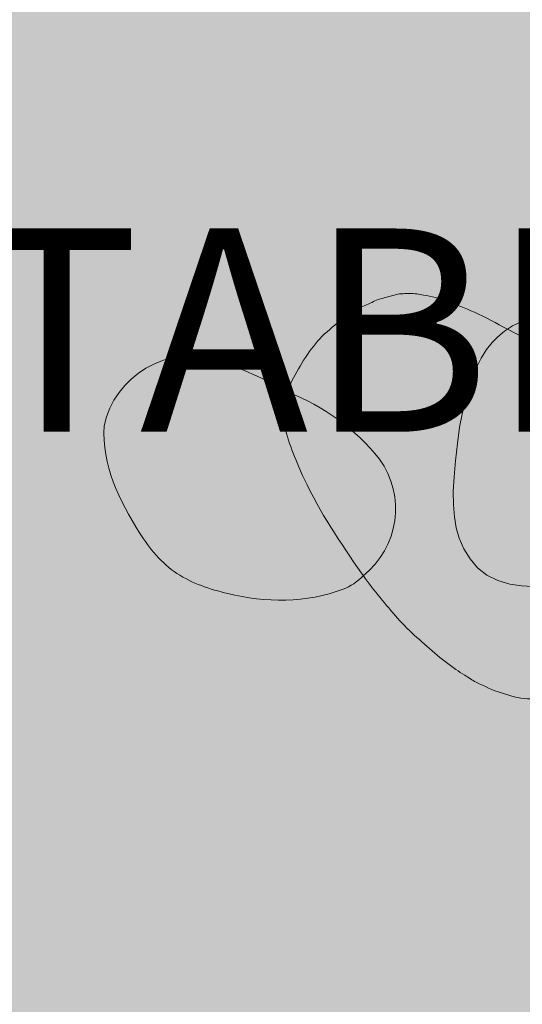
# Model space of a CAD drawing. Units: inches. Extents: x -466983 to 1020, y 324 to 318697.
# Tile 14 of 97: x 767 to 782, y 452 to 482. Entities that reach past the tile are written whole.
import ezdxf

# ---------------------------------------------------------------- set-up
doc = ezdxf.new("R2010")
doc.units = ezdxf.units.IN
doc.header["$MEASUREMENT"] = 0
for name, color, linetype, lineweight in [('A-ANNO-DIMS', 2, 'Continuous', 18), ('A-FLOR-PATT', 252, 'Continuous', 13), ('A-FURN', 8, 'Continuous', 18)]:
    doc.layers.add(name, color=color, linetype=linetype, lineweight=lineweight)
doc.layers.add('K-Hatch', color=7, linetype='Continuous')
doc.styles.get("Standard").update_dxf_attribs({"font": 'arial.ttf'})
doc.dimstyles.get("Standard").update_dxf_attribs({"dimtxt": 6, "dimasz": 4, "dimexe": 3, "dimexo": 3, "dimgap": 0.09, "dimtad": 0, "dimtih": 1, "dimtoh": 1, "dimdec": 1, "dimzin": 0, "dimdsep": 46, "dimlunit": 3, "dimtxsty": 'Standard', "dimcen": 0.09, "dimadec": 0, "dimazin": 0, "dimtfac": 1, "dimtdec": 1, "dimtofl": 0, "dimtmove": 0, "dimatfit": 3, "dimfxl": 1, "dimtolj": 1, "dimtzin": 0, "dimarcsym": 0})

# ---------------------------------------------------------------- blocks, each defined once
blk = doc.blocks.new('CBV_08')
at = {"layer": 'K-Hatch'}
h = blk.add_hatch(color=256, dxfattribs=at)
h.dxf.hatch_style = 1
h.set_gradient(color1=(254, 240, 205), color2=(128, 128, 128), name='INVSPHERICAL')
edge = h.paths.add_edge_path()
edge.add_line((-64.79138966518599, 606.517606906063), (-20.81558270819153, 613.546301131098))
edge.add_line((-20.81558270819153, 613.546301131098), (24.32122939205357, 618.7037140054739))
edge.add_line((24.32122939205357, 618.7037140054739), (72.9395138398707, 622.3681759726226))
edge.add_line((72.9395138398707, 622.3681759726226), (121.1548466474654, 624.3855799447387))
edge.add_line((121.1548466474654, 624.3855799447387), (138.0302417780076, 624.4468206786386))
edge.add_spline(control_points=[(138.030241778006, 624.4468206786399), (115.3772409944233, 641.9915953521052), (92.47135367460055, 659.1511423863225), (69.51887429453404, 676.0537172357374)], knot_values=[4, 4, 4, 4, 4.295360820963978, 4.295360820963978, 4.295360820963978, 4.295360820963978], degree=3, periodic=0)
edge.add_spline(control_points=[(69.51887429453404, 676.0537172357374), (30.70506570139173, 704.6353462207347), (-11.00942055295832, 728.169079543611), (-55.2545562042194, 747.1615514590061)], knot_values=[3, 3, 3, 3, 4, 4, 4, 4], degree=3, periodic=0)
edge.add_spline(control_points=[(-55.2545562042194, 747.1615514590061), (-74.79123232152574, 755.5682692145741), (-96.04647521982929, 763.3373296114872), (-116.9964348293704, 766.9793317465076)], knot_values=[2, 2, 2, 2, 3, 3, 3, 3], degree=3, periodic=0)
edge.add_spline(control_points=[(-116.9964348293704, 766.9793317465076), (-129.2025380821412, 769.1194214050287), (-142.5645676213296, 773.3606469692544), (-154.9264209480295, 773.6061289003395)], knot_values=[1, 1, 1, 1, 2, 2, 2, 2], degree=3, periodic=0)
edge.add_spline(control_points=[(-154.9264209480295, 773.6061289003395), (-167.4825847303998, 773.8346847966089), (-180.0262076523775, 774.0748753660085), (-192.5707367616394, 774.2908904018253)], knot_values=[0, 0, 0, 0, 1, 1, 1, 1], degree=3, periodic=0)
edge.add_spline(control_points=[(-192.5707367616394, 774.2908904018253), (-216.7903187338359, 770.7925997045726), (-242.1798570897642, 768.0523435204025), (-264.5867622564817, 757.3685138498098)], knot_values=[36, 36, 36, 36, 37, 37, 37, 37], degree=3, periodic=0)
edge.add_spline(control_points=[(-264.5867622564817, 757.3685138498098), (-290.3942303536148, 745.0932751511913), (-313.89668970258, 731.3395900077523), (-338.2351472893185, 716.2736138413578)], knot_values=[35, 35, 35, 35, 36, 36, 36, 36], degree=3, periodic=0)
edge.add_spline(control_points=[(-338.2351472893185, 716.2736138413578), (-347.9610121955609, 710.3073903524285), (-356.8308795163155, 702.311797133457), (-365.9258992755765, 695.4140709847092)], knot_values=[34, 34, 34, 34, 35, 35, 35, 35], degree=3, periodic=0)
edge.add_spline(control_points=[(-365.9258992755765, 695.4140709847092), (-373.6755679803298, 689.5311341952842), (-381.8593443391417, 684.0155071080865), (-388.9610960997213, 677.3335799996441)], knot_values=[33, 33, 33, 33, 34, 34, 34, 34], degree=3, periodic=0)
edge.add_spline(control_points=[(-388.9610960997213, 677.3335799996441), (-406.729828736248, 660.5687764882745), (-425.2306395907051, 644.6182227184574), (-440.976605720263, 625.9497812193016)], knot_values=[32, 32, 32, 32, 33, 33, 33, 33], degree=3, periodic=0)
edge.add_spline(control_points=[(-440.976605720263, 625.9497812193016), (-457.3792275295688, 606.5554590512905), (-473.1295788334953, 588.0929626809404), (-486.9148680956839, 566.8332397690232)], knot_values=[31, 31, 31, 31, 32, 32, 32, 32], degree=3, periodic=0)
edge.add_spline(control_points=[(-486.9148680956839, 566.8332397690232), (-500.9035296869967, 545.3148354868893), (-513.6024407896599, 524.6196286704019), (-525.3262890138119, 501.8421701200517)], knot_values=[30, 30, 30, 30, 31, 31, 31, 31], degree=3, periodic=0)
edge.add_spline(control_points=[(-525.3262890138119, 501.8421701200517), (-537.3020063965502, 478.4810197776608), (-547.0309200097087, 455.6408885381519), (-556.5438888201876, 431.1343120964632)], knot_values=[29, 29, 29, 29, 30, 30, 30, 30], degree=3, periodic=0)
edge.add_spline(control_points=[(-556.5438888201876, 431.1343120964632), (-560.0561410925272, 422.0421443586014), (-562.5749468278061, 413.9416423962169), (-564.7102456379196, 404.4468236496863)], knot_values=[28, 28, 28, 28, 29, 29, 29, 29], degree=3, periodic=0)
edge.add_spline(control_points=[(-564.7102456379196, 404.4468236496863), (-567.4125701169521, 392.4191567675519), (-572.8198041777047, 378.6287482230977), (-573.2577841897707, 366.2983199287131)], knot_values=[27, 27, 27, 27, 28, 28, 28, 28], degree=3, periodic=0)
edge.add_spline(control_points=[(-573.2577841897707, 366.2983199287131), (-574.1266404775649, 341.5040448117628), (-575.304810477535, 317.8228961875114), (-572.5731788796527, 293.1720708856777)], knot_values=[26, 26, 26, 26, 27, 27, 27, 27], degree=3, periodic=0)
edge.add_spline(control_points=[(-572.5731788796527, 293.1720708856777), (-569.7888110403416, 268.3134880803485), (-564.7375575475141, 244.8346089123782), (-559.2381346902381, 220.39476018934)], knot_values=[25, 25, 25, 25, 26, 26, 26, 26], degree=3, periodic=0)
edge.add_spline(control_points=[(-559.2381346902381, 220.39476018934), (-554.0809714274053, 197.480834403956), (-542.3092427474018, 175.0331508067478), (-531.2413547152225, 154.4759812873775)], knot_values=[24, 24, 24, 24, 25, 25, 25, 25], degree=3, periodic=0)
edge.add_spline(control_points=[(-531.2413547152225, 154.4759812873775), (-519.403151221251, 132.5099959863458), (-505.0181011074143, 113.2568476545442), (-490.3048531095534, 93.07143623794889)], knot_values=[23, 23, 23, 23, 24, 24, 24, 24], degree=3, periodic=0)
edge.add_spline(control_points=[(-490.3048531095534, 93.07143623794889), (-483.3509117323826, 83.53853831289995), (-473.9591893545564, 75.10052898437368), (-465.9930630307915, 66.41333744620022)], knot_values=[22, 22, 22, 22, 23, 23, 23, 23], degree=3, periodic=0)
edge.add_spline(control_points=[(-465.9930630307915, 66.41333744620022), (-459.6548847536303, 59.50604190370757), (-453.604240079321, 52.35532441345128), (-446.6990045201653, 46.04411576107247)], knot_values=[21, 21, 21, 21, 22, 22, 22, 22], degree=3, periodic=0)
edge.add_spline(control_points=[(-446.6990045201653, 46.04411576107247), (-428.9342653979526, 29.76310043132924), (-411.702585725752, 12.82420009659779), (-392.8242828237105, -2.167033131417724)], knot_values=[20, 20, 20, 20, 21, 21, 21, 21], degree=3, periodic=0)
edge.add_spline(control_points=[(-392.8242828237105, -2.167033131417724), (-354.8913445483756, -32.28926142704006), (-316.7323476472791, -63.48518125932298), (-274.7460244996744, -87.8401222976778)], knot_values=[19, 19, 19, 19, 20, 20, 20, 20], degree=3, periodic=0)
edge.add_spline(control_points=[(-274.7460244996744, -87.8401222976778), (-234.955018883325, -110.9307710282837), (-195.1384319972665, -133.6252783222554), (-153.3221455000149, -152.8648495164187)], knot_values=[18.05838940751118, 18.05838940751118, 18.05838940751118, 18.05838940751118, 19, 19, 19, 19], degree=3, periodic=0)
edge.add_arc((49.86677919520497, -261.3467220115906), 230.3346603941012, 65.03867317360732, 151.9023938369816, ccw=False)
edge.add_arc((-129.2812027509484, -567.9672323098254), 584.8490139284039, 31.48529429409882, 61.80224086708262, ccw=False)
edge.add_spline(control_points=[(369.4629719679939, -262.512461063759), (382.1414530141528, -256.3251174853196), (394.4447979650791, -248.8650481942471), (404.7778651476567, -240.2778876530971)], knot_values=[14, 14, 14, 14, 14.63913933614759, 14.63913933614759, 14.63913933614759, 14.63913933614759], degree=3, periodic=0)
edge.add_spline(control_points=[(404.7778651476567, -240.2778876530971), (441.3463170029883, -209.9220561231274), (479.5607774255643, -176.9890874269773), (505.1149959804917, -136.2702973715255)], knot_values=[13, 13, 13, 13, 14, 14, 14, 14], degree=3, periodic=0)
edge.add_spline(control_points=[(505.1149959804917, -136.2702973715255), (530.8465989563576, -95.34027082563227), (553.1783362005974, -52.43077807973225), (563.4385548192388, -4.759509566932706)], knot_values=[12, 12, 12, 12, 13, 13, 13, 13], degree=3, periodic=0)
edge.add_spline(control_points=[(563.4385548192388, -4.759509566932706), (565.9042695621922, 6.768626796916919), (569.9291446497102, 18.87987190328147), (570.8906849512443, 30.64596147769623)], knot_values=[11, 11, 11, 11, 12, 12, 12, 12], degree=3, periodic=0)
edge.add_spline(control_points=[(570.8906849512443, 30.64596147769623), (571.9830393682371, 44.61021222987381), (573.0870284582799, 58.56192212158965), (574.2026522214603, 72.50109115288376)], knot_values=[10, 10, 10, 10, 11, 11, 11, 11], degree=3, periodic=0)
edge.add_spline(control_points=[(574.2026522214603, 72.50109115288376), (575.1354860527229, 84.147209246937), (571.5785970058952, 97.43839810787028), (570.3069263480158, 109.0461015825534)], knot_values=[9, 9, 9, 9, 10, 10, 10, 10], degree=3, periodic=0)
edge.add_spline(control_points=[(570.3069263480158, 109.0461015825534), (569.0514212999572, 120.7621418644797), (562.8733150448844, 133.2316224966274), (559.2635756073307, 144.46698481903)], knot_values=[8, 8, 8, 8, 9, 9, 9, 9], degree=3, periodic=0)
edge.add_spline(control_points=[(559.2635756073307, 144.46698481903), (552.8041526084727, 164.6093172202094), (542.0082472319502, 184.6721018205611), (531.3772170289905, 202.9977269928053)], knot_values=[7, 7, 7, 7, 8, 8, 8, 8], degree=3, periodic=0)
edge.add_spline(control_points=[(531.3772170289905, 202.9977269928053), (517.9036702272736, 226.2233812246626), (504.23704229505, 248.1731693027863), (488.9372065676455, 270.147861726345)], knot_values=[6, 6, 6, 6, 7, 7, 7, 7], degree=3, periodic=0)
edge.add_spline(control_points=[(488.9372065676455, 270.147861726345), (469.8533160771787, 297.5925618256764), (449.2354871813461, 323.7854631127206), (427.5991442464021, 349.1168170453524)], knot_values=[5.661323372545377, 5.661323372545377, 5.661323372545377, 5.661323372545377, 6, 6, 6, 6], degree=3, periodic=0)
edge.add_line((427.5991442463698, 349.1168170453909), (423.9747477541691, 340.6014840513798))
edge.add_line((423.9747477541691, 340.6014840513798), (412.808934445699, 320.4232347897252))
edge.add_line((412.808934445699, 320.4232347897252), (399.8478922482787, 302.2360483816345))
edge.add_line((399.8478922482787, 302.2360483816345), (384.0539504526838, 283.8987745838916))
edge.add_line((384.0539504526838, 283.8987745838916), (364.156960334922, 265.3525599682313))
edge.add_line((364.156960334922, 265.3525599682313), (338.8501862328868, 246.4446252659333))
edge.add_line((338.8501862328868, 246.4446252659333), (310.9097775188589, 228.7884705858413))
edge.add_line((310.9097775188589, 228.7884705858413), (283.0295862930982, 213.9660194435388))
edge.add_line((283.0295862930982, 213.9660194435388), (254.7738784127343, 200.7279684327768))
edge.add_line((254.7738784127343, 200.7279684327768), (225.6329419192077, 187.8474673446376))
edge.add_line((225.6329419192077, 187.8474673446376), (191.8889572177454, 174.7078000831396))
edge.add_line((191.8889572177454, 174.7078000831396), (149.8016515162934, 160.6182727369141))
edge.add_line((149.8016515162934, 160.6182727369141), (105.1969968870397, 147.0988901004634))
edge.add_line((105.1969968870397, 147.0988901004634), (63.83901812491513, 135.5187941953463))
edge.add_line((63.83901812491513, 135.5187941953463), (25.49254533584696, 126.4341179003361))
edge.add_line((25.49254533584696, 126.4341179003361), (-10.07718940434142, 120.2958416550874))
edge.add_line((-10.07718940434142, 120.2958416550874), (-42.72473563698878, 116.9709475091298))
edge.add_line((-42.72473563698878, 116.9709475091298), (-72.3050448734702, 116.4315699508456))
edge.add_line((-72.3050448734702, 116.4315699508456), (-101.0374515771664, 119.3513048962898))
edge.add_line((-101.0374515771664, 119.3513048962898), (-131.2036394586584, 126.3580379276175))
edge.add_line((-131.2036394586584, 126.3580379276175), (-160.9794301176425, 137.5525283719678))
edge.add_line((-160.9794301176425, 137.5525283719678), (-188.5011510736637, 153.1124205142454))
edge.add_line((-188.5011510736637, 153.1124205142454), (-212.640701596012, 173.826418601469))
edge.add_line((-212.640701596012, 173.826418601469), (-232.358494479731, 200.5908844919054))
edge.add_line((-232.358494479731, 200.5908844919054), (-247.523586420544, 230.3767474503167))
edge.add_line((-247.523586420544, 230.3767474503167), (-257.9655400341414, 260.2318216988527))
edge.add_line((-257.9655400341414, 260.2318216988527), (-265.4557098397616, 290.3624857707295))
edge.add_line((-265.4557098397616, 290.3624857707295), (-271.7375848450154, 321.1201666878492))
edge.add_line((-271.7375848450154, 321.1201666878492), (-275.6639202339554, 353.4897398345838))
edge.add_line((-275.6639202339554, 353.4897398345838), (-276.0791517338637, 388.5101103857555))
edge.add_line((-276.0791517338637, 388.5101103857555), (-273.5370652017862, 421.6149104247238))
edge.add_line((-273.5370652017862, 421.6149104247238), (-268.5769107842041, 448.1525676207844))
edge.add_line((-268.5769107842041, 448.1525676207844), (-261.6384708784151, 470.9065601562581))
edge.add_line((-261.6384708784151, 470.9065601562581), (-253.1640330542267, 492.5722546573825))
edge.add_line((-253.1640330542267, 492.5722546573825), (-243.7239572843808, 512.1755070152225))
edge.add_line((-243.7239572843808, 512.1755070152225), (-233.7319264845262, 528.6461440779487))
edge.add_line((-233.7319264845262, 528.6461440779487), (-222.3769051199757, 543.1922739391771))
edge.add_line((-222.3769051199757, 543.1922739391771), (-208.8220953469844, 556.9737891860306))
edge.add_line((-208.8220953469844, 556.9737891860306), (-193.021478215143, 569.1041619425226))
edge.add_line((-193.021478215143, 569.1041619425226), (-174.8604692728239, 578.6033404621488))
edge.add_line((-174.8604692728239, 578.6033404621488), (-148.974808163095, 587.3334464585154))
edge.add_line((-148.974808163095, 587.3334464585154), (-109.8867626335099, 597.2110334055883))
edge.add_line((-109.8867626335099, 597.2110334055883), (-64.79138966518599, 606.517606906063))
edge = h.paths.add_edge_path()
edge.add_spline(control_points=[(370.7740806031818, -764.2232780453443), (495.6890758351384, -715.2963272131716), (556.220503779916, -553.3182213584847), (490.446566071276, -435.7530750287375)], knot_values=[8, 8, 8, 8, 9, 9, 9, 9], degree=3, periodic=0)
edge.add_spline(control_points=[(490.446566071276, -435.7530750287375), (456.6036438010944, -375.2577718323315), (415.1029492433028, -316.5884105847386), (369.4629719679963, -262.5124610637619)], knot_values=[7.311196124620593, 7.311196124620593, 7.311196124620593, 7.311196124620593, 8, 8, 8, 8], degree=3, periodic=0)
edge.add_spline(control_points=[(369.4629719679939, -262.512461063759), (362.3046500995046, -266.0058603664158), (355.0267431928314, -269.0935430374898), (347.9163499642475, -271.749297319148)], knot_values=[14.63913933614759, 14.63913933614759, 14.63913933614759, 14.63913933614759, 15, 15, 15, 15], degree=3, periodic=0)
edge.add_spline(control_points=[(347.9163499642475, -271.749297319148), (326.0039438658589, -279.8975602920933), (303.3824373709524, -287.9103008374319), (279.5615269071152, -286.9084633086364)], knot_values=[15, 15, 15, 15, 16, 16, 16, 16], degree=3, periodic=0)
edge.add_spline(control_points=[(279.5615269071152, -286.9084633086364), (229.2836666359237, -284.8301893640761), (180.9876047627497, -274.1228849437854), (132.3314510729999, -261.719522663721)], knot_values=[16, 16, 16, 16, 17, 17, 17, 17], degree=3, periodic=0)
edge.add_spline(control_points=[(132.3314510729999, -261.719522663721), (36.00218488264568, -237.1675315866047), (-55.01748718155226, -196.9089215037244), (-145.5195049805604, -156.4034104861035)], knot_values=[17, 17, 17, 17, 18, 18, 18, 18], degree=3, periodic=0)
edge.add_spline(control_points=[(-145.5195049805604, -156.4034104861035), (-148.1283883267314, -155.2376615191636), (-150.7291115936745, -154.0578980778492), (-153.3221455000149, -152.8648495164187)], knot_values=[18, 18, 18, 18, 18.05838940751119, 18.05838940751119, 18.05838940751119, 18.05838940751119], degree=3, periodic=0)
edge.add_spline(control_points=[(-274.7460244996744, -87.8401222976778), (-234.955018883325, -110.9307710282837), (-195.1384319972665, -133.6252783222554), (-153.3221455000149, -152.8648495164187)], knot_values=[18.05838940751118, 18.05838940751118, 18.05838940751118, 18.05838940751118, 19, 19, 19, 19], degree=3, periodic=0)
edge.add_spline(control_points=[(-153.3221455000146, -152.8648495164185), (-165.9784966016575, -171.5529182496635), (-175.5394621391003, -191.9432962999195), (-179.1806174456121, -212.6958639215733)], knot_values=[4, 4, 4, 4, 4.452928820811951, 4.452928820811951, 4.452928820811951, 4.452928820811951], degree=3, periodic=0)
edge.add_spline(control_points=[(-179.1806174456121, -212.6958639215733), (-197.3592812184049, -316.3139201192631), (-177.1543255416015, -424.9652546180692), (-133.8373497511472, -520.2132515876334)], knot_values=[3, 3, 3, 3, 4, 4, 4, 4], degree=3, periodic=0)
edge.add_spline(control_points=[(-133.8373497511472, -520.2132515876334), (-113.812089820012, -564.2398904196585), (-89.6918054411924, -609.8211379272631), (-55.59549708207282, -644.6841850643032)], knot_values=[2, 2, 2, 2, 3, 3, 3, 3], degree=3, periodic=0)
edge.add_spline(control_points=[(-55.59549708207282, -644.6841850643032), (-21.01697530070465, -680.0323447207999), (24.09120381830348, -705.467011840744), (69.80118293775217, -723.3015190900511)], knot_values=[1, 1, 1, 1, 2, 2, 2, 2], degree=3, periodic=0)
edge.add_spline(control_points=[(69.80118293775217, -723.3015190900511), (165.7170699927976, -760.7319885564399), (268.3409267343543, -790.7494799387347), (370.7740806031818, -764.2232780453443)], knot_values=[0, 0, 0, 0, 1, 1, 1, 1], degree=3, periodic=0)
h = blk.add_hatch(color=256, dxfattribs=at)
h.dxf.hatch_style = 1
h.set_gradient(color1=(237, 238, 153), color2=(128, 128, 128), name='INVSPHERICAL')
h.paths.add_polyline_path([(138.030241777993, 624.4468206786385), (121.1548466474651, 624.3855799447387), (72.93951383987078, 622.3681759726226), (24.32122939205266, 618.7037140054739), (-20.81558270819135, 613.5463011310981), (-64.79138966518634, 606.517606906063), (-109.8867626335099, 597.2110334055883), (-148.9748081630947, 587.3334464585154), (-174.8604692728237, 578.6033404621488), (-193.0214782151431, 569.1041619425226), (-208.8220953469843, 556.9737891860306), (-222.3769051199757, 543.192273939177), (-233.7319264845262, 528.6461440779487), (-243.7239572843807, 512.1755070152223), (-253.1640330542266, 492.5722546573828), (-261.6384708784152, 470.906560156258), (-268.5769107842041, 448.1525676207845), (-273.5370652017862, 421.6149104247238), (-276.0791517338637, 388.5101103857553), (-275.6639202339554, 353.4897398345842), (-271.7375848450154, 321.120166687849), (-265.4557098397615, 290.3624857707285), (-257.9655400341414, 260.2318216988531), (-247.5235864205439, 230.376747450317), (-232.3584944797308, 200.5908844919054), (-212.6407015960119, 173.826418601469), (-188.501151073664, 153.1124205142455), (-160.9794301176417, 137.5525283719673), (-131.203639458659, 126.3580379276176), (-101.0374515771665, 119.3513048962899), (-72.30504487347056, 116.4315699508456), (-42.72473563698999, 116.9709475091296), (-10.07718940434079, 120.2958416550876), (25.49254533584675, 126.4341179003363), (63.83901812491291, 135.5187941953455), (105.1969968870418, 147.0988901004643), (149.8016515162908, 160.6182727369133), (191.8889572177462, 174.707800083141), (225.6329419192069, 187.8474673446376), (254.7738784127325, 200.7279684327774), (283.0295862930968, 213.9660194435376), (310.9097775188592, 228.7884705858409), (338.8501862328868, 246.4446252659339), (364.1569603349224, 265.3525599682311), (384.0539504526849, 283.8987745838923), (399.8478922482773, 302.2360483816343), (412.8089344456993, 320.4232347897255), (423.9747477541696, 340.6014840513813), (427.5991442463708, 349.1168170453934, 0.0927646108411709)])
h.paths.add_polyline_path([(388.7752655456738, 558.0333432889242), (367.1251050861341, 577.3131219875615), (341.0917552188349, 593.091853727265), (309.7395752683536, 604.7890359364814), (275.6176774626967, 613.1902790132755), (241.3915530672843, 619.1185842334983), (205.1930145804382, 622.8339579509642), (165.1625959267279, 624.545283871213), (138.0302417779927, 624.4468206786386, -0.0927646108411711), (427.599144246371, 349.116817045393), (434.2528920744103, 364.7494550682643), (441.5708112205049, 390.8300374801888), (443.8189600989302, 416.8173475254692), (441.0824212141471, 444.9881519235453), (433.4579056388776, 477.5510538625714), (421.7913917255954, 509.5471564446192), (406.9263526543529, 535.9294512156752)])
edge = h.paths.add_edge_path()
edge.add_arc((49.86677919520502, -261.3467220115905), 230.3346603941012, 65.0386731736079, 151.9023938369817)
edge.add_spline(control_points=[(-153.3221455000149, -152.8648495164187), (-150.7291115936745, -154.0578980778492), (-148.1283883267314, -155.2376615191636), (-145.5195049805604, -156.4034104861035)], knot_values=[18, 18, 18, 18, 18.05838940751118, 18.05838940751118, 18.05838940751118, 18.05838940751118], degree=3, periodic=0)
edge.add_spline(control_points=[(-145.5195049805604, -156.4034104861035), (-55.01748718155226, -196.9089215037244), (36.00218488264568, -237.1675315866047), (132.3314510729999, -261.719522663721)], knot_values=[17, 17, 17, 17, 18, 18, 18, 18], degree=3, periodic=0)
edge.add_spline(control_points=[(132.3314510729999, -261.719522663721), (180.9876047627497, -274.1228849437854), (229.2836666359237, -284.8301893640761), (279.5615269071152, -286.9084633086364)], knot_values=[16, 16, 16, 16, 17, 17, 17, 17], degree=3, periodic=0)
edge.add_spline(control_points=[(279.5615269071152, -286.9084633086364), (303.3824373709524, -287.9103008374319), (326.0039438658589, -279.8975602920933), (347.9163499642475, -271.749297319148)], knot_values=[15, 15, 15, 15, 16, 16, 16, 16], degree=3, periodic=0)
edge.add_spline(control_points=[(347.9163499642475, -271.749297319148), (355.0267431928314, -269.0935430374898), (362.3046500995046, -266.0058603664158), (369.4629719679939, -262.512461063759)], knot_values=[14.63913933614759, 14.63913933614759, 14.63913933614759, 14.63913933614759, 15, 15, 15, 15], degree=3, periodic=0)
edge.add_arc((-129.2812027509481, -567.9672323098252), 584.8490139284037, 31.48529429409889, 61.80224086708276)
edge = h.paths.add_edge_path()
edge.add_spline(control_points=[(490.446566071276, -435.7530750287375), (456.6036438010944, -375.2577718323315), (415.1029492433028, -316.5884105847386), (369.4629719679963, -262.5124610637619)], knot_values=[7.311196124620593, 7.311196124620593, 7.311196124620593, 7.311196124620593, 8, 8, 8, 8], degree=3, periodic=0)
edge.add_spline(control_points=[(369.4629719679939, -262.512461063759), (362.3046500995046, -266.0058603664158), (355.0267431928314, -269.0935430374898), (347.9163499642475, -271.749297319148)], knot_values=[14.63913933614759, 14.63913933614759, 14.63913933614759, 14.63913933614759, 15, 15, 15, 15], degree=3, periodic=0)
edge.add_spline(control_points=[(347.9163499642475, -271.749297319148), (326.0039438658589, -279.8975602920933), (303.3824373709524, -287.9103008374319), (279.5615269071152, -286.9084633086364)], knot_values=[15, 15, 15, 15, 16, 16, 16, 16], degree=3, periodic=0)
edge.add_spline(control_points=[(279.5615269071152, -286.9084633086364), (229.2836666359237, -284.8301893640761), (180.9876047627497, -274.1228849437854), (132.3314510729999, -261.719522663721)], knot_values=[16, 16, 16, 16, 17, 17, 17, 17], degree=3, periodic=0)
edge.add_spline(control_points=[(132.3314510729999, -261.719522663721), (36.00218488264568, -237.1675315866047), (-55.01748718155226, -196.9089215037244), (-145.5195049805604, -156.4034104861035)], knot_values=[17, 17, 17, 17, 18, 18, 18, 18], degree=3, periodic=0)
edge.add_spline(control_points=[(-145.5195049805604, -156.4034104861035), (-148.1283883267314, -155.2376615191636), (-150.7291115936745, -154.0578980778492), (-153.3221455000149, -152.8648495164187)], knot_values=[18, 18, 18, 18, 18.05838940751119, 18.05838940751119, 18.05838940751119, 18.05838940751119], degree=3, periodic=0)
edge.add_spline(control_points=[(-274.7460244996744, -87.8401222976778), (-234.955018883325, -110.9307710282837), (-195.1384319972665, -133.6252783222554), (-153.3221455000149, -152.8648495164187)], knot_values=[18.05838940751118, 18.05838940751118, 18.05838940751118, 18.05838940751118, 19, 19, 19, 19], degree=3, periodic=0)
edge.add_spline(control_points=[(-153.3221455000146, -152.8648495164185), (-165.9784966016575, -171.5529182496635), (-175.5394621391003, -191.9432962999195), (-179.1806174456121, -212.6958639215733)], knot_values=[4, 4, 4, 4, 4.452928820811951, 4.452928820811951, 4.452928820811951, 4.452928820811951], degree=3, periodic=0)
edge.add_spline(control_points=[(-179.1806174456121, -212.6958639215733), (-197.3592812184049, -316.3139201192631), (-177.1543255416015, -424.9652546180692), (-133.8373497511472, -520.2132515876334)], knot_values=[3, 3, 3, 3, 4, 4, 4, 4], degree=3, periodic=0)
edge.add_spline(control_points=[(-133.8373497511472, -520.2132515876334), (-113.812089820012, -564.2398904196585), (-89.6918054411924, -609.8211379272631), (-55.59549708207282, -644.6841850643032)], knot_values=[2, 2, 2, 2, 3, 3, 3, 3], degree=3, periodic=0)
edge.add_spline(control_points=[(-55.59549708207282, -644.6841850643032), (-21.01697530070465, -680.0323447207999), (24.09120381830348, -705.467011840744), (69.80118293775217, -723.3015190900511)], knot_values=[1, 1, 1, 1, 2, 2, 2, 2], degree=3, periodic=0)
edge.add_spline(control_points=[(69.80118293775217, -723.3015190900511), (165.7170699927976, -760.7319885564399), (268.3409267343543, -790.7494799387347), (370.7740806031818, -764.2232780453443)], knot_values=[0, 0, 0, 0, 1, 1, 1, 1], degree=3, periodic=0)
edge.add_spline(control_points=[(370.7740806031818, -764.2232780453443), (495.6890758351384, -715.2963272131716), (556.220503779916, -553.3182213584847), (490.446566071276, -435.7530750287375)], knot_values=[8, 8, 8, 8, 9, 9, 9, 9], degree=3, periodic=0)
for points in [[(441.570811220505, 390.8300374801887), (443.8189600989301, 416.8173475254692)], [(434.25289207441, 364.7494550682635), (441.570811220505, 390.8300374801887)], [(423.9747477541698, 340.6014840513811), (434.25289207441, 364.7494550682635)], [(399.8478922482775, 302.2360483816341), (412.8089344456986, 320.4232347897254)], [(412.8089344456986, 320.4232347897254), (423.9747477541698, 340.6014840513811)], [(384.0539504526844, 283.8987745838916), (399.8478922482775, 302.2360483816341)], [(-265.4557098397615, 290.3624857707295), (-257.9655400341414, 260.2318216988527)], [(338.8501862328869, 246.4446252659339), (364.1569603349219, 265.3525599682311)], [(364.1569603349219, 265.3525599682311), (384.0539504526844, 283.8987745838916)], [(-257.9655400341414, 260.2318216988527), (-247.523586420544, 230.3767474503169)], [(310.9097775188586, 228.7884705858409), (338.8501862328869, 246.4446252659339)], [(-247.523586420544, 230.3767474503169), (-232.358494479731, 200.5908844919053)], [(254.7738784127307, 200.7279684327772), (283.0295862930963, 213.9660194435377)], [(254.7738784127307, 200.7279684327772), (283.0295862930963, 213.9660194435377)], [(283.0295862930963, 213.9660194435377), (310.9097775188586, 228.7884705858409)], [(-232.358494479731, 200.5908844919053), (-212.6407015960119, 173.8264186014688)], [(191.8889572177452, 174.7078000831401), (225.6329419192064, 187.8474673446375)], [(225.6329419192064, 187.8474673446375), (254.7738784127307, 200.7279684327772)], [(227.5366038028462, 188.7158703379876), (226.0668814761759, 188.0793281267473)], [(-212.6407015960119, 173.8264186014688), (-188.5011510736638, 153.1124205142454)], [(105.1969968870419, 147.0988901004642), (149.801651516291, 160.6182727369136)], [(149.801651516291, 160.6182727369136), (191.8889572177452, 174.7078000831401)], [(149.801651516291, 160.6182727369136), (191.8889572177452, 174.7078000831401)], [(-188.5011510736638, 153.1124205142454), (-160.9794301176423, 137.5525283719674)], [(-160.9794301176423, 137.5525283719674), (-131.2036394586591, 126.3580379276176)], [(25.49254533584667, 126.4341179003362), (63.83901812491444, 135.5187941953458)], [(63.83901812491444, 135.5187941953458), (105.1969968870419, 147.0988901004642)], [(-131.2036394586591, 126.3580379276176), (-101.0374515771671, 119.3513048962899)], [(-101.0374515771671, 119.3513048962899), (-72.30504487347002, 116.4315699508455)], [(-72.30504487347002, 116.4315699508455), (-42.72473563698963, 116.9709475091298)], [(-42.72473563698963, 116.9709475091298), (-10.07718940434074, 120.2958416550876)], [(-10.07718940434074, 120.2958416550876), (25.49254533584667, 126.4341179003362)]]:
    blk.add_lwpolyline(points)
at = {"ltscale": 150}
for centre, radius, start, end in [((-452.8125879761916, -286.8889818885906), 1086.106898289845, 35.84419107960195, 57.04360384091717), ((49.86677919520502, -261.3467220115905), 230.3346603941012, 65.03867317409953, 151.902393837143), ((-129.2812027509478, -567.9672323098252), 584.8490139284035, 31.48529429389016, 61.8022408668417)]:
    blk.add_arc(centre, radius, start, end, dxfattribs=at)
for points, knots in [([(427.5991442464021, 349.1168170453524), (449.2354871813461, 323.7854631127206), (469.8533160771787, 297.5925618256764), (488.9372065676455, 270.147861726345), (504.23704229505, 248.1731693027863), (517.9036702272736, 226.2233812246626), (531.3772170289905, 202.9977269928053), (542.0082472319502, 184.6721018205611), (552.8041526084727, 164.6093172202094), (559.2635756073307, 144.46698481903), (562.8733150448844, 133.2316224966274), (569.0514212999572, 120.7621418644797), (570.3069263480158, 109.0461015825534), (571.5785970058952, 97.43839810787028), (575.1354860527229, 84.147209246937), (574.2026522214603, 72.50109115288376), (573.0870284582799, 58.56192212158965), (571.9830393682371, 44.61021222987381), (570.8906849512443, 30.64596147769623), (569.9291446497102, 18.87987190328147), (565.9042695621922, 6.768626796916919), (563.4385548192388, -4.759509566932706), (553.1783362005974, -52.43077807973225), (530.8465989563576, -95.34027082563227), (505.1149959804917, -136.2702973715255), (479.5607774255643, -176.9890874269773), (441.3463170029883, -209.9220561231274), (404.7778651476567, -240.2778876530971), (388.6107062854592, -253.7133938963976), (367.6203352994073, -264.3897966927667), (347.9163499642475, -271.749297319148), (326.0039438658589, -279.8975602920933), (303.3824373709524, -287.9103008374319), (279.5615269071152, -286.9084633086364), (229.2836666359237, -284.8301893640761), (180.9876047627497, -274.1228849437854), (132.3314510729999, -261.719522663721), (36.00218488264568, -237.1675315866047), (-55.01748718155226, -196.9089215037244), (-145.5195049805604, -156.4034104861035), (-190.20026913579, -136.4383343425139), (-232.487572934069, -112.3626254585375), (-274.7460244996744, -87.8401222976778), (-316.7323476472791, -63.48518125932298), (-354.8913445483756, -32.28926142704006), (-392.8242828237105, -2.167033131417724), (-411.702585725752, 12.82420009659779), (-428.9342653979526, 29.76310043132924), (-446.6990045201653, 46.04411576107247), (-453.604240079321, 52.35532441345128), (-459.6548847536303, 59.50604190370757), (-465.9930630307915, 66.41333744620022), (-473.9591893545564, 75.10052898437368), (-483.3509117323826, 83.53853831289995), (-490.3048531095534, 93.07143623794889), (-505.0181011074143, 113.2568476545442), (-519.403151221251, 132.5099959863458), (-531.2413547152225, 154.4759812873775), (-542.3092427474018, 175.0331508067478), (-554.0809714274053, 197.480834403956), (-559.2381346902381, 220.39476018934), (-564.7375575475141, 244.8346089123782), (-569.7888110403416, 268.3134880803485), (-572.5731788796527, 293.1720708856777), (-575.304810477535, 317.8228961875114), (-574.1266404775649, 341.5040448117628), (-573.2577841897707, 366.2983199287131), (-572.8198041777047, 378.6287482230977), (-567.4125701169521, 392.4191567675519), (-564.7102456379196, 404.4468236496863), (-562.5749468278061, 413.9416423962169), (-560.0561410925272, 422.0421443586014), (-556.5438888201876, 431.1343120964632), (-547.0309200097087, 455.6408885381519), (-537.3020063965502, 478.4810197776608), (-525.3262890138119, 501.8421701200517), (-513.6024407896599, 524.6196286704019), (-500.9035296869967, 545.3148354868893), (-486.9148680956839, 566.8332397690232), (-473.1295788334953, 588.0929626809404), (-457.3792275295688, 606.5554590512905), (-440.976605720263, 625.9497812193016), (-425.2306395907051, 644.6182227184574), (-406.729828736248, 660.5687764882745), (-388.9610960997213, 677.3335799996441), (-381.8593443391417, 684.0155071080865), (-373.6755679803298, 689.5311341952842), (-365.9258992755765, 695.4140709847092), (-356.8308795163155, 702.311797133457), (-347.9610121955609, 710.3073903524285), (-338.2351472893185, 716.2736138413578), (-313.89668970258, 731.3395900077523), (-290.3942303536148, 745.0932751511913), (-264.5867622564817, 757.3685138498098), (-242.1798570897642, 768.0523435204025), (-216.7903187338359, 770.7925997045726), (-192.5707367616394, 774.2908904018253)], [5.661323372545377, 5.661323372545377, 5.661323372545377, 5.661323372545377, 6, 6, 6, 7, 7, 7, 8, 8, 8, 9, 9, 9, 10, 10, 10, 11, 11, 11, 12, 12, 12, 13, 13, 13, 14, 14, 14, 15, 15, 15, 16, 16, 16, 17, 17, 17, 18, 18, 18, 19, 19, 19, 20, 20, 20, 21, 21, 21, 22, 22, 22, 23, 23, 23, 24, 24, 24, 25, 25, 25, 26, 26, 26, 27, 27, 27, 28, 28, 28, 29, 29, 29, 30, 30, 30, 31, 31, 31, 32, 32, 32, 33, 33, 33, 34, 34, 34, 35, 35, 35, 36, 36, 36, 37, 37, 37, 37]), ([(370.7740806031818, -764.2232780453443), (268.3409267343543, -790.7494799387347), (165.7170699927976, -760.7319885564399), (69.80118293775217, -723.3015190900511), (24.09120381830348, -705.467011840744), (-21.01697530070465, -680.0323447207999), (-55.59549708207282, -644.6841850643032), (-89.6918054411924, -609.8211379272631), (-113.812089820012, -564.2398904196585), (-133.8373497511472, -520.2132515876334), (-177.1543255416015, -424.9652546180692), (-197.3592812184049, -316.3139201192631), (-179.1806174456121, -212.6958639215733), (-175.5394621391003, -191.9432962999195), (-165.9784966016575, -171.5529182496635), (-153.3221455000146, -152.8648495164185)], [0, 0, 0, 0, 1, 1, 1, 2, 2, 2, 3, 3, 3, 4, 4, 4, 4.452928820811951, 4.452928820811951, 4.452928820811951, 4.452928820811951]), ([(369.4629719679963, -262.5124610637619), (415.1029492433028, -316.5884105847386), (456.6036438010944, -375.2577718323315), (490.446566071276, -435.7530750287375), (556.220503779916, -553.3182213584847), (495.6890758351384, -715.2963272131716), (370.7740806031818, -764.2232780453443)], [7.311196124620593, 7.311196124620593, 7.311196124620593, 7.311196124620593, 8, 8, 8, 9, 9, 9, 9])]:
    blk.add_open_spline(points, degree=3, knots=knots)
blk = doc.blocks.new('Garden Sofa')
at = {"extrusion": (0, 0, -1)}
blk.add_ellipse((2450.434344520113, 828.9172181338074), major_axis=(18.680571335226, -14.92282860552713), ratio=0.8335261636002053, start_param=9.234639352962448, end_param=10.28481875168741, dxfattribs=at)
at = {"xscale": -0.0109740885734132, "yscale": 0.0109740885734132, "zscale": 0.0109740885734132, "rotation": 280.5267845499334}
blk.add_blockref('CBV_08', (2451.372776762163, 829.7810777878433), dxfattribs=at)
blk = doc.blocks.new('*D113')
at = {"layer": 'A-ANNO-DIMS', "color": 0, "lineweight": -2, "transparency": 16777216}
for p, q in [((704.7099345407843, 504.6522237351473), (709.5248847709719, 509.4132675549068)), ((710.2041170385384, 504.4596180389745), (736.3194883324882, 478.0485582412536)), ((736.4502266725144, 472.5525555338968), (741.2651769027019, 477.3135993536564)), ((739.1319487513783, 475.2042540394889), (741.9444091702684, 472.359949837724)), ((741.9444091702684, 472.359949837724), (745.9444091702684, 472.359949837724))]:
    blk.add_line(p, q, dxfattribs=at)
at = {"layer": 'A-ANNO-DIMS', "color": 0, "transparency": 16777216}
for points in [[(710.6781677388324, 504.9283614421228), (709.7300663382443, 503.9908746358262), (707.3916566196483, 507.3039222407393)], [(736.7935390327824, 478.5173016444019), (735.8454376321941, 477.5798148381053), (739.1319487513783, 475.2042540394889)]]:
    blk.add_solid(points, dxfattribs=at)
at = {"layer": 'Defpoints', "color": 0, "transparency": 16777216}
for p in [(702.5767063894607, 502.5428784209798), (739.1319487513783, 475.2042540394889), (734.3169985211908, 470.4432102197293)]:
    blk.add_point(p, dxfattribs=at)
at = {"layer": 'A-ANNO-DIMS', "color": 0, "transparency": 16777216, "insert": (783.5016670147431, 472.359949837724), "char_height": 6, "attachment_point": 5}
blk.add_mtext('\\A1;TEA TABLE SET 45', dxfattribs=at)

msp = doc.modelspace()

# ---------------------------------------------------------------- hatches: boundary and pattern name
at = {"layer": 'A-FLOR-PATT', "transparency": 33554661}
h = msp.add_hatch(color=256, dxfattribs=at)
h.dxf.hatch_style = 1
h.set_gradient(color1=(19, 155, 72), color2=(0, 107, 0), name='CYLINDER')
h.paths.add_polyline_path([(813.8056775209042, 503.9377328184218), (730.8056775209043, 503.9377328184218), (730.8056775209043, 424.9377328184218), (612.8056775209042, 424.9377328184218), (612.8056775209042, 415.9377328184218), (442.8056775209042, 415.9377328184218), (442.8056775209042, 368.9377328184219), (813.8056775209042, 368.9377328184219)])
h.paths.add_polyline_path([(771.7959187717115, 407.069553802904), (783.7959187717115, 407.069553802904), (783.7959187717115, 371.069553802904), (771.7959187717115, 371.069553802904)], flags=16)
h.paths.add_polyline_path([(755.7959187717115, 407.069553802904), (755.7959187717115, 371.069553802904), (743.7959187717114, 371.069553802904), (743.7959187717114, 407.069553802904)], flags=16)
h.paths.add_polyline_path([(769.7959187717115, 404.069553802904), (769.7959187717115, 374.069553802904), (757.7959187717115, 374.069553802904), (757.7959187717115, 404.069553802904)], flags=16)
h.paths.add_polyline_path([(785.7959187717114, 404.069553802904), (797.7959187717114, 404.069553802904), (797.7959187717114, 374.069553802904), (785.7959187717114, 374.069553802904)], flags=16)
h.paths.add_polyline_path([(741.7959187717115, 404.069553802904), (741.7959187717115, 374.069553802904), (729.7959187717115, 374.069553802904), (729.7959187717115, 404.069553802904)], flags=16)
h.paths.add_polyline_path([(799.7959187717115, 407.069553802904), (811.7959187717115, 407.069553802904), (811.7959187717115, 371.069553802904), (799.7959187717115, 371.069553802904)], flags=16)
h.paths.add_polyline_path([(727.7959187717115, 407.069553802904), (727.7959187717115, 371.069553802904), (715.7959187717115, 371.069553802904), (715.7959187717115, 407.069553802904)], flags=16)
h.paths.add_polyline_path([(713.7959187717115, 404.069553802904), (713.7959187717115, 374.069553802904), (701.7959187717115, 374.069553802904), (701.7959187717115, 404.069553802904)], flags=16)
h.paths.add_polyline_path([(699.7959187717115, 407.069553802904), (699.7959187717115, 371.069553802904), (687.7959187717115, 371.069553802904), (687.7959187717115, 407.069553802904)], flags=16)
h.paths.add_polyline_path([(685.7959187717114, 404.069553802904), (685.7959187717114, 374.069553802904), (673.7959187717115, 374.069553802904), (673.7959187717115, 404.069553802904)], flags=16)
h.paths.add_polyline_path([(671.7959187717115, 407.069553802904), (671.7959187717115, 371.069553802904), (659.7959187717115, 371.069553802904), (659.7959187717115, 407.069553802904)], flags=16)
h.paths.add_polyline_path([(657.7959187717115, 404.069553802904), (657.7959187717115, 374.069553802904), (645.7959187717115, 374.069553802904), (645.7959187717115, 404.069553802904)], flags=16)
h.paths.add_polyline_path([(643.7959187717114, 407.069553802904), (643.7959187717114, 371.069553802904), (631.7959187717114, 371.069553802904), (631.7959187717114, 407.069553802904)], flags=16)
h.paths.add_polyline_path([(629.7959187717115, 404.069553802904), (629.7959187717115, 374.069553802904), (617.7959187717115, 374.069553802904), (617.7959187717115, 404.069553802904)], flags=16)
h.paths.add_polyline_path([(615.7959187717115, 407.069553802904), (615.7959187717115, 371.069553802904), (603.7959187717115, 371.069553802904), (603.7959187717115, 407.069553802904)], flags=16)
h.paths.add_polyline_path([(601.7959187717115, 404.069553802904), (601.7959187717115, 374.069553802904), (589.7959187717114, 374.069553802904), (589.7959187717114, 404.069553802904)], flags=16)
at = {"layer": 'A-FLOR-PATT'}
h = msp.add_hatch(dxfattribs=at)
h.set_pattern_fill('GRASS', color=256, scale=6)
h.set_pattern_definition([(90, (-1212.413693079869, -290.0350025265127), (-4.242640685999999, 4.242640685999999), [1.125, -7.360281377999999]), (45, (-1212.413693079869, -290.0350025265127), (-4.242640687119285, 4.242640687119285), [1.125, -4.875]), (135, (-1212.413693079869, -290.0350025265127), (-4.242640687119285, -4.242640687119284), [1.125, -4.875])])
h.paths.add_polyline_path([(813.8056775209042, 503.9377328184218), (730.8056775209043, 503.9377328184218), (730.8056775209043, 424.9377328184218), (612.8056775209042, 424.9377328184218), (612.8056775209042, 415.9377328184218), (442.8056775209042, 415.9377328184218), (442.8056775209042, 368.9377328184219), (813.8056775209042, 368.9377328184219)])
h.paths.add_polyline_path([(589.7959187717114, 404.069553802904), (601.7959187717115, 404.069553802904), (601.7959187717115, 374.069553802904), (589.7959187717114, 374.069553802904)], flags=16)
h.paths.add_polyline_path([(603.7959187717115, 407.069553802904), (615.7959187717115, 407.069553802904), (615.7959187717115, 371.069553802904), (603.7959187717115, 371.069553802904)], flags=16)
h.paths.add_polyline_path([(617.7959187717115, 404.069553802904), (629.7959187717115, 404.069553802904), (629.7959187717115, 374.069553802904), (617.7959187717115, 374.069553802904)], flags=16)
h.paths.add_polyline_path([(631.7959187717114, 407.069553802904), (643.7959187717114, 407.069553802904), (643.7959187717114, 371.069553802904), (631.7959187717114, 371.069553802904)], flags=16)
h.paths.add_polyline_path([(645.7959187717115, 404.069553802904), (657.7959187717115, 404.069553802904), (657.7959187717115, 374.069553802904), (645.7959187717115, 374.069553802904)], flags=16)
h.paths.add_polyline_path([(659.7959187717115, 407.069553802904), (671.7959187717115, 407.069553802904), (671.7959187717115, 371.069553802904), (659.7959187717115, 371.069553802904)], flags=16)
h.paths.add_polyline_path([(673.7959187717115, 404.069553802904), (685.7959187717114, 404.069553802904), (685.7959187717114, 374.069553802904), (673.7959187717115, 374.069553802904)], flags=16)
h.paths.add_polyline_path([(687.7959187717115, 407.069553802904), (699.7959187717115, 407.069553802904), (699.7959187717115, 371.069553802904), (687.7959187717115, 371.069553802904)], flags=16)
h.paths.add_polyline_path([(701.7959187717115, 404.069553802904), (713.7959187717115, 404.069553802904), (713.7959187717115, 374.069553802904), (701.7959187717115, 374.069553802904)], flags=16)
h.paths.add_polyline_path([(715.7959187717115, 407.069553802904), (727.7959187717115, 407.069553802904), (727.7959187717115, 371.069553802904), (715.7959187717115, 371.069553802904)], flags=16)
h.paths.add_polyline_path([(729.7959187717115, 404.069553802904), (741.7959187717115, 404.069553802904), (741.7959187717115, 374.069553802904), (729.7959187717115, 374.069553802904)], flags=16)
h.paths.add_polyline_path([(743.7959187717114, 407.069553802904), (755.7959187717115, 407.069553802904), (755.7959187717115, 371.069553802904), (743.7959187717114, 371.069553802904)], flags=16)
h.paths.add_polyline_path([(757.7959187717115, 404.069553802904), (769.7959187717115, 404.069553802904), (769.7959187717115, 374.069553802904), (757.7959187717115, 374.069553802904)], flags=16)
h.paths.add_polyline_path([(771.7959187717115, 407.069553802904), (783.7959187717115, 407.069553802904), (783.7959187717115, 371.069553802904), (771.7959187717115, 371.069553802904)], flags=16)
h.paths.add_polyline_path([(785.7959187717114, 404.069553802904), (797.7959187717114, 404.069553802904), (797.7959187717114, 374.069553802904), (785.7959187717114, 374.069553802904)], flags=16)
h.paths.add_polyline_path([(799.7959187717115, 407.069553802904), (811.7959187717115, 407.069553802904), (811.7959187717115, 371.069553802904), (799.7959187717115, 371.069553802904)], flags=16)

# ---------------------------------------------------------------- block references
at = {"layer": 'A-FURN'}
msp.add_blockref('Garden Sofa', (-1672.699650965823, -362.7106367544016), dxfattribs=at)

# ---------------------------------------------------------------- dimensions: what is measured, and where the dimension line sits
at = {"layer": 'A-ANNO-DIMS'}
dim = msp.add_linear_dim(base=(739.1319487513783, 475.2042540394889), p1=(702.5767063894607, 502.5428784209797), p2=(734.3169985211907, 470.4432102197293), angle=314.6774666770457, text='TEA TABLE SET <>', dimstyle='Standard', override={"dimdec": 0, "dimlfac": 1, "dimrnd": 0, "dimzin": 0, "dimdsep": 46, "dimlunit": 2}, dxfattribs=at)
dim.commit()
dim.dimension.update_dxf_attribs({"geometry": '*D113', "text_midpoint": (783.5016670147431, 472.359949837724)})

doc.saveas('drawing.dxf')
